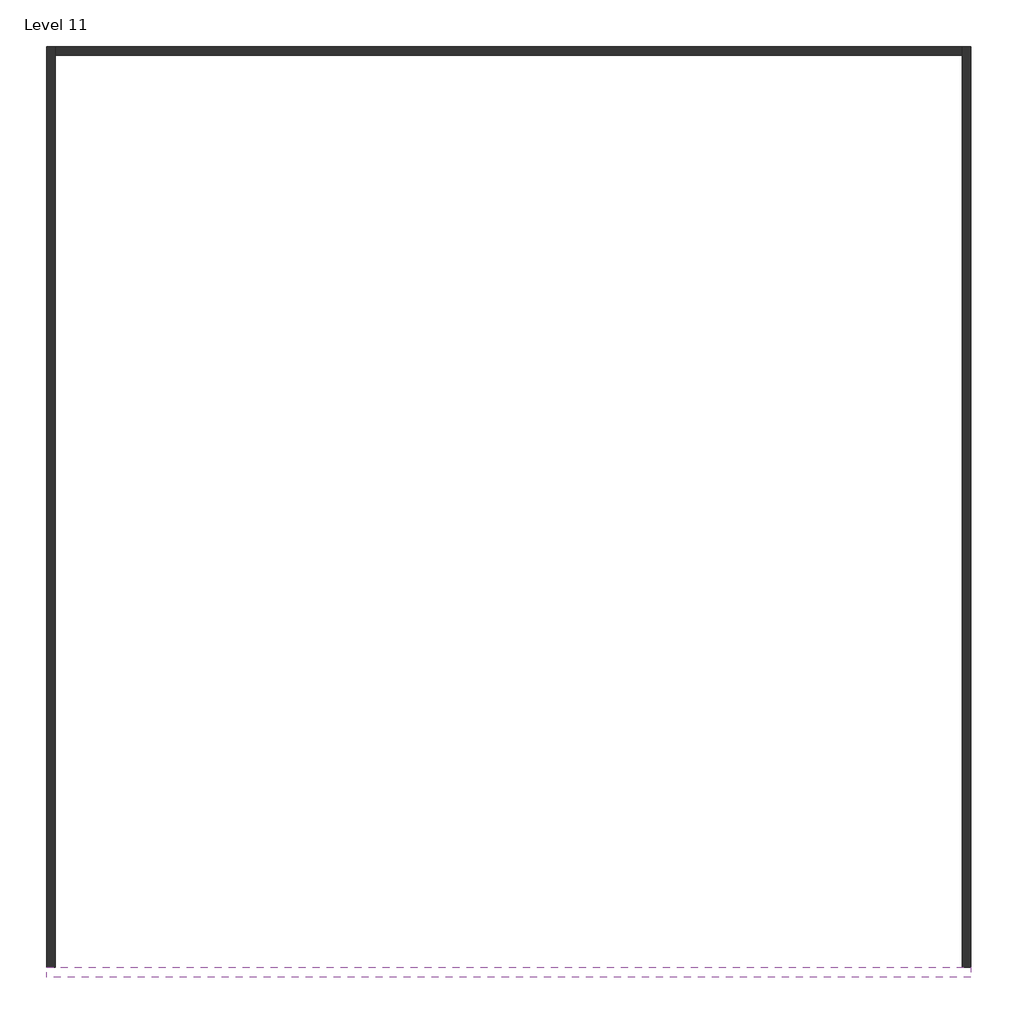
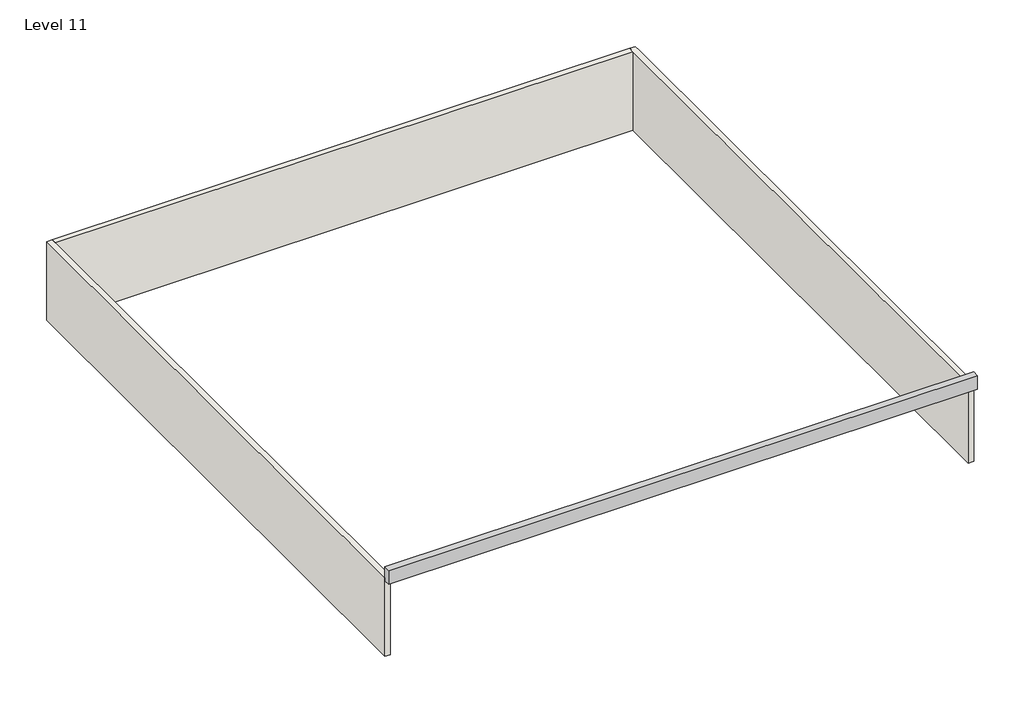
# One storey: 3 walls, 1 proxy.
"""IFC4 building model written with IfcOpenShell, lengths in millimetres."""

from ifc_helpers import new_model, si_unit, frame, origin, place, context, project, spatial, polyline, outline, extrude, faceted_brep, transform, mapped, element, save
from components import generic_models_8_generic_models_8_a9945552

model = new_model("IFC4")

# Units and contexts
model_context = context("Model", 3, world=origin())
ifc_project = project(units=[si_unit("LENGTHUNIT", "METRE", prefix="MILLI")], contexts=[model_context])

# Site, building, storey
site = spatial("IfcSite", under=ifc_project)
building = spatial("IfcBuilding", under=site)
storey = spatial("IfcBuildingStorey", under=building, Name="Level 11", Elevation=16383.0)

# Proxy
placement = place(None, origin())
generic_models_8_generic_models_8_shape = generic_models_8_generic_models_8_a9945552(model_context)
element("IfcBuildingElementProxy", 1, Name="Generic Models 8 : Generic Models 8", ObjectType="Generic Models 8 : Generic Models 8", at=placement, inside=storey, context=model_context, shape_type="MappedRepresentation", body=[
    mapped(generic_models_8_generic_models_8_shape, transform((0.0, 0.0, 0.0), x_axis=(1.0, 0.0, 0.0), y_axis=(0.0, 1.0, 0.0), z_axis=(0.0, 0.0, 1.0))),
])

# Walls
element("IfcWall", 2, ObjectType="outer wall", at=placement, inside=storey, context=model_context, shape_type="Brep", body=[
    faceted_brep([(-8731.5629849, -3682.5004242, 16383.0), (-8731.5629849, 17551.8995758, 16383.0), (-8731.5629849, 17755.0995758, 16383.0), (-8731.5629849, 17755.0995758, 19431.0), (-8731.5629849, 17551.8995758, 19431.0), (-8731.5629849, -3682.5004242, 19431.0), (-8934.7629849, -3682.5004242, 16383.0), (-8934.7629849, -3682.5004242, 19431.0), (-8934.7629849, 17551.8995758, 19431.0), (-8934.7629849, 17755.0995758, 19431.0), (-8934.7629849, 17755.0995758, 16383.0)], [[[0, 1, 2, 3, 4, 5]], [[6, 7, 8, 9, 10]], [[2, 1, 0, 6, 10]], [[0, 5, 7, 6]], [[5, 4, 3, 9, 8, 7]], [[3, 2, 10, 9]]]),
])
element("IfcWall", 3, ObjectType="outer wall", at=placement, inside=storey, context=model_context, shape_type="Brep", body=[
    faceted_brep([(12604.4370151, -3682.5004242, 16383.0), (12604.4370151, 17755.0995758, 16383.0), (12604.4370151, 17755.0995758, 19431.0), (12604.4370151, 17551.8995758, 19431.0), (12604.4370151, -3682.5004242, 19431.0), (12401.2370151, -3682.5004242, 16383.0), (12401.2370151, -3682.5004242, 19431.0), (12401.2370151, 17551.8995758, 19431.0), (12401.2370151, 17755.0995758, 19431.0), (12401.2370151, 17755.0995758, 16383.0), (12401.2370151, 17551.8995758, 16383.0)], [[[0, 1, 2, 3, 4]], [[5, 6, 7, 8, 9, 10]], [[1, 0, 5, 10, 9]], [[0, 4, 6, 5]], [[4, 3, 2, 8, 7, 6]], [[2, 1, 9, 8]]]),
])
element("IfcWall", 4, ObjectType="outer wall", at=placement, inside=storey, context=model_context, shape_type="SweptSolid", body=[
    extrude(outline(polyline([(12401.2370151, 17551.8995758), (-8731.5629849, 17551.8995758), (-8731.5629849, 17755.0995758), (12401.2370151, 17755.0995758), (12401.2370151, 17551.8995758)])), frame((0.0, 0.0, 16383.0), z_axis=(0.0, 0.0, 1.0), x_axis=(1.0, 0.0, 0.0)), (0.0, 0.0, 1.0), 3048.0),
])

save(model, "model.ifc")

# Revit data of these elements
# Type "outer wall"
#   Assembly Code = "B2010"
#   Layers, outside or top first: 0' - 8" "Copper" (function 1)
# Element 1 (IfcBuildingElementProxy, "Generic Models 8 : Generic Models 8")
#   Phase Created = New Construction
# Elements 2, 3, 4 (IfcWall, "outer wall")
#   Top Offset = 0' - 0"
#   Base Offset = 0' - 0"
#   Unconnected Height = 10' - 0"
#   wall height = 10' - 0"
#   Phase Created = New Construction
#   Base Constraint = Level 11
#   Materials on its faces: "Copper"
# Materials
#   "Copper": class "Metal", colour RGB 0 0 0, transparency 0, Description = "Copper, matte finish", Cost = 0
